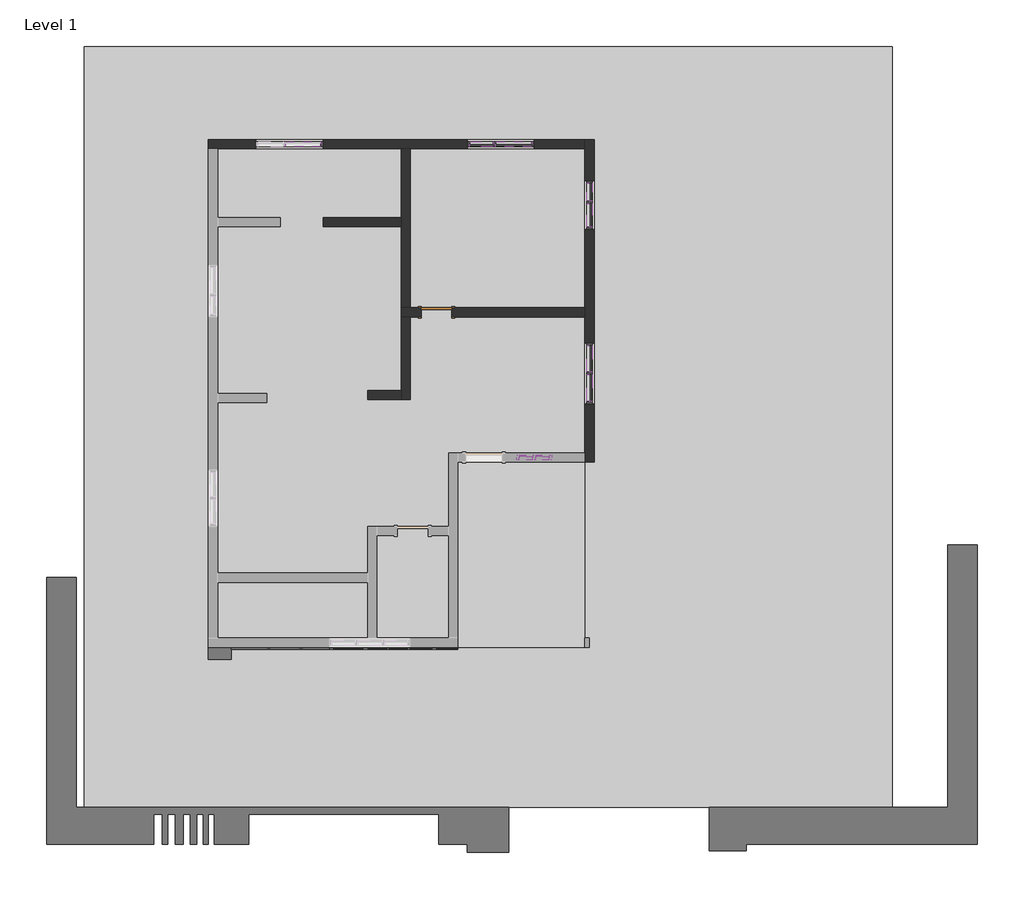
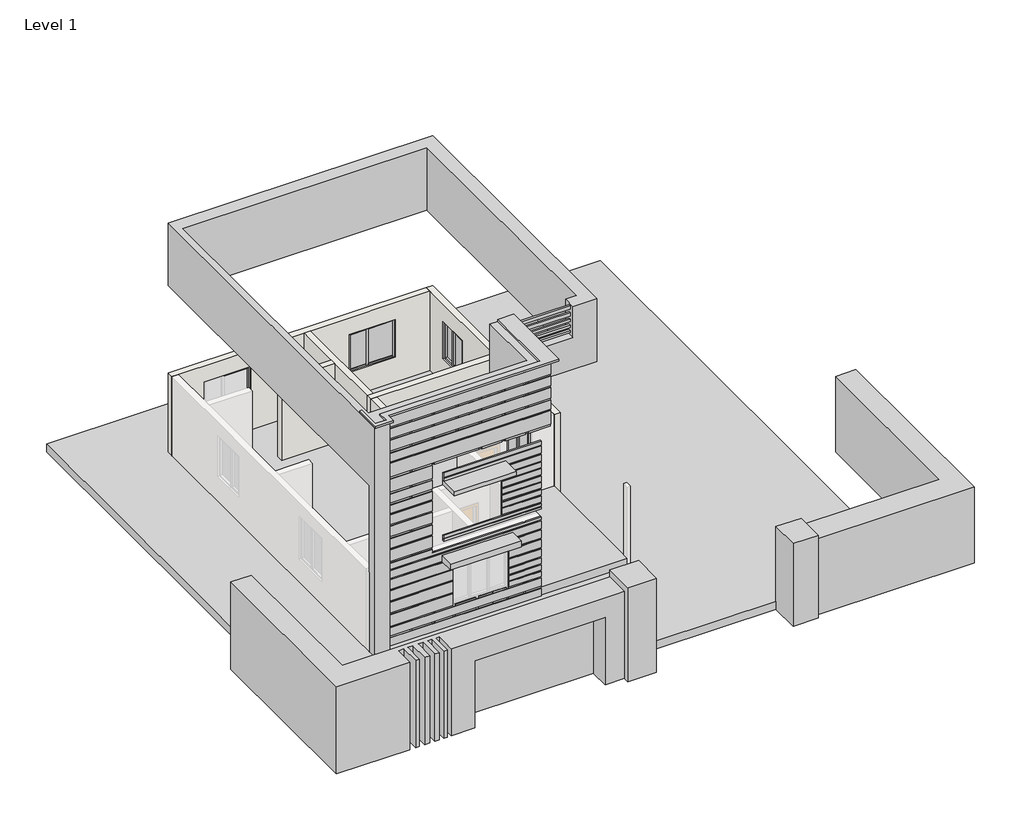
# One storey, part 2 of 2: 30 members, 8 plates, 7 walls, 2 proxies, 1 door.
"""IFC4 building model written with IfcOpenShell, lengths in millimetres."""

from ifc_helpers import new_model, si_unit, origin, origin_with_axes, place, context, project, spatial, polyline, outline, extrude, faceted_brep, transform, mapped, element, save
from components import generic_models_1_generic_models_1_0bf7fa05, generic_models_3_generic_models_3_b56d3d43, generic_models_3_generic_models_3_92db7db1, door_a1484949, member_9f7b9c5b, member_75cd65a6, member_fc57e1ce, member_c33c434a, member_7824d57a, member_cb331184, member_6fb4a552, member_e5d39754, member_b85431e0, member_e39930a5, member_f1f71bde, member_0700671e, member_9dfa5507, member_024c663a, member_55cf8d67, system_panel_glazed_7b9e2e16, system_panel_glazed_a4d37703, system_panel_glazed_197f3525, system_panel_glazed_f1c06e49, system_panel_glazed_593bec76, system_panel_glazed_469e0694

model = new_model("IFC4")

# Units and contexts
model_context = context("Model", 3, world=origin())
ifc_project = project(units=[si_unit("LENGTHUNIT", "METRE", prefix="MILLI")], contexts=[model_context])

# Site, building, storey
site = spatial("IfcSite", under=ifc_project)
building = spatial("IfcBuilding", under=site)
storey = spatial("IfcBuildingStorey", under=building, Name="Level 1", Elevation=0.0)

# Proxies
placement = place(None, origin())
generic_models_1_generic_models_1_shape = generic_models_1_generic_models_1_0bf7fa05(model_context)
element("IfcBuildingElementProxy", 1, Name="Generic Models 1 : Generic Models 1", ObjectType="Generic Models 1 : Generic Models 1", at=placement, inside=storey, context=model_context, shape_type="MappedRepresentation", body=[
    mapped(generic_models_1_generic_models_1_shape, transform((0.0, 0.0, 0.0), x_axis=(1.0, 0.0, 0.0), y_axis=(0.0, 1.0, 0.0), z_axis=(0.0, 0.0, 1.0))),
])
generic_models_3_generic_models_3_shape = generic_models_3_generic_models_3_b56d3d43(model_context)
generic_models_3_generic_models_3_2_shape = generic_models_3_generic_models_3_92db7db1(model_context)
element("IfcBuildingElementProxy", 2, Name="Generic Models 3 : Generic Models 3", ObjectType="Generic Models 3 : Generic Models 3", at=placement, inside=storey, context=model_context, shape_type="MappedRepresentation", body=[
    mapped(generic_models_3_generic_models_3_shape, transform((0.0, 0.0, 0.0), x_axis=(1.0, 0.0, 0.0), y_axis=(0.0, 1.0, 0.0), z_axis=(0.0, 0.0, 1.0))),
    mapped(generic_models_3_generic_models_3_2_shape, transform((0.0, 0.0, 0.0), x_axis=(1.0, 0.0, 0.0), y_axis=(0.0, 1.0, 0.0), z_axis=(0.0, 0.0, 1.0))),
])

# Door
door_shape = door_a1484949(model_context)
element("IfcDoor", 3, ObjectType="Single-Flush : 30\" x 80\"", at=placement, inside=storey, context=model_context, shape_type="MappedRepresentation", body=[
    mapped(door_shape, transform((-12850.1628107, -5472.3642965, 0.0), x_axis=(1.0, 0.0, 0.0), y_axis=(0.0, 1.0, 0.0), z_axis=(0.0, 0.0, 1.0))),
])

# Members
member_shape = member_9f7b9c5b(model_context)
element("IfcMember", 4, ObjectType="Rectangular Mullion : 2.5\" x 5\" rectangular", at=placement, inside=storey, context=model_context, shape_type="MappedRepresentation", body=[
    mapped(member_shape, transform((-10446.6878107, -9091.8642965, 2736.7021457), x_axis=(0.0, 0.0, 1.0), y_axis=(0.0, -1.0, 0.0), z_axis=(1.0, 0.0, 0.0))),
])
element("IfcMember", 5, ObjectType="Rectangular Mullion : 2.5\" x 5\" rectangular", at=placement, inside=storey, context=model_context, shape_type="MappedRepresentation", body=[
    mapped(member_shape, transform((-10037.1128107, -9091.8642965, 2736.7021457), x_axis=(0.0, 0.0, 1.0), y_axis=(0.0, -1.0, 0.0), z_axis=(1.0, 0.0, 0.0))),
])
member_2_shape = member_75cd65a6(model_context)
element("IfcMember", 6, ObjectType="Rectangular Mullion : 2.5\" x 5\" rectangular", at=placement, inside=storey, context=model_context, shape_type="MappedRepresentation", body=[
    mapped(member_2_shape, transform((-10414.9378107, -9091.8642965, 1249.7277266), x_axis=(1.0, 0.0, 0.0), y_axis=(0.0, -1.0, 0.0), z_axis=(0.0, 0.0, -1.0))),
])
element("IfcMember", 7, ObjectType="Rectangular Mullion : 2.5\" x 5\" rectangular", at=placement, inside=storey, context=model_context, shape_type="MappedRepresentation", body=[
    mapped(member_shape, transform((-10383.1878107, -9091.8642965, 1249.7277266), x_axis=(0.0, 0.0, -1.0), y_axis=(0.0, -1.0, 0.0), z_axis=(-1.0, 0.0, 0.0))),
])
element("IfcMember", 8, ObjectType="Rectangular Mullion : 2.5\" x 5\" rectangular", at=placement, inside=storey, context=model_context, shape_type="MappedRepresentation", body=[
    mapped(member_shape, transform((-10792.7628107, -9091.8642965, 1249.7277266), x_axis=(0.0, 0.0, -1.0), y_axis=(0.0, -1.0, 0.0), z_axis=(-1.0, 0.0, 0.0))),
])
member_3_shape = member_fc57e1ce(model_context)
element("IfcMember", 9, ObjectType="Rectangular Mullion : 2.5\" x 5\" rectangular", at=placement, inside=storey, context=model_context, shape_type="MappedRepresentation", body=[
    mapped(member_3_shape, transform((-10856.2628107, -9091.8642965, 2736.7021457), x_axis=(-1.0, 0.0, 0.0), y_axis=(0.0, -1.0, 0.0), z_axis=(0.0, 0.0, 1.0))),
])
element("IfcMember", 10, ObjectType="Rectangular Mullion : 2.5\" x 5\" rectangular", at=placement, inside=storey, context=model_context, shape_type="MappedRepresentation", body=[
    mapped(member_3_shape, transform((-9973.6128107, -9091.8642965, 1249.7277266), x_axis=(1.0, 0.0, 0.0), y_axis=(0.0, -1.0, 0.0), z_axis=(0.0, 0.0, -1.0))),
])
member_4_shape = member_c33c434a(model_context)
element("IfcMember", 11, ObjectType="Rectangular Mullion : 2.5\" x 5\" rectangular", at=placement, inside=storey, context=model_context, shape_type="MappedRepresentation", body=[
    mapped(member_4_shape, transform((-9040.1628107, -7028.1142965, 1098.1511575), x_axis=(0.0, 0.0, -1.0), y_axis=(-1.0, 0.0, 0.0), z_axis=(0.0, 1.0, 0.0))),
])
element("IfcMember", 12, ObjectType="Rectangular Mullion : 2.5\" x 5\" rectangular", at=placement, inside=storey, context=model_context, shape_type="MappedRepresentation", body=[
    mapped(member_4_shape, transform((-9040.1628107, -6297.8642965, 1098.1511575), x_axis=(0.0, 0.0, -1.0), y_axis=(-1.0, 0.0, 0.0), z_axis=(0.0, 1.0, 0.0))),
])
member_5_shape = member_7824d57a(model_context)
element("IfcMember", 13, ObjectType="Rectangular Mullion : 2.5\" x 5\" rectangular", at=placement, inside=storey, context=model_context, shape_type="MappedRepresentation", body=[
    mapped(member_5_shape, transform((-9040.1628107, -6996.3642965, 1098.1511575), x_axis=(0.0, -1.0, 0.0), y_axis=(-1.0, 0.0, 0.0), z_axis=(0.0, 0.0, -1.0))),
])
element("IfcMember", 14, ObjectType="Rectangular Mullion : 2.5\" x 5\" rectangular", at=placement, inside=storey, context=model_context, shape_type="MappedRepresentation", body=[
    mapped(member_4_shape, transform((-9040.1628107, -6964.6142965, 2379.6118359), x_axis=(0.0, 0.0, 1.0), y_axis=(-1.0, 0.0, 0.0), z_axis=(0.0, -1.0, 0.0))),
])
element("IfcMember", 15, ObjectType="Rectangular Mullion : 2.5\" x 5\" rectangular", at=placement, inside=storey, context=model_context, shape_type="MappedRepresentation", body=[
    mapped(member_4_shape, transform((-9040.1628107, -7694.8642965, 2379.6118359), x_axis=(0.0, 0.0, 1.0), y_axis=(-1.0, 0.0, 0.0), z_axis=(0.0, -1.0, 0.0))),
])
member_6_shape = member_cb331184(model_context)
element("IfcMember", 16, ObjectType="Rectangular Mullion : 2.5\" x 5\" rectangular", at=placement, inside=storey, context=model_context, shape_type="MappedRepresentation", body=[
    mapped(member_6_shape, transform((-9040.1628107, -6234.3642965, 2379.6118359), x_axis=(0.0, 1.0, 0.0), y_axis=(-1.0, 0.0, 0.0), z_axis=(0.0, 0.0, 1.0))),
])
element("IfcMember", 17, ObjectType="Rectangular Mullion : 2.5\" x 5\" rectangular", at=placement, inside=storey, context=model_context, shape_type="MappedRepresentation", body=[
    mapped(member_6_shape, transform((-9040.1628107, -7758.3642965, 1098.1511575), x_axis=(0.0, -1.0, 0.0), y_axis=(-1.0, 0.0, 0.0), z_axis=(0.0, 0.0, -1.0))),
])
member_7_shape = member_6fb4a552(model_context)
element("IfcMember", 18, ObjectType="Rectangular Mullion : 2.5\" x 5\" rectangular", at=placement, inside=storey, context=model_context, shape_type="MappedRepresentation", body=[
    mapped(member_7_shape, transform((-9040.1628107, -2259.2642965, 941.1853188), x_axis=(0.0, 0.0, -1.0), y_axis=(-1.0, 0.0, 0.0), z_axis=(0.0, 1.0, 0.0))),
])
member_8_shape = member_e5d39754(model_context)
element("IfcMember", 19, ObjectType="Rectangular Mullion : 2.5\" x 5\" rectangular", at=placement, inside=storey, context=model_context, shape_type="MappedRepresentation", body=[
    mapped(member_8_shape, transform((-9040.1628107, -2760.9142965, 941.1853188), x_axis=(0.0, 0.0, -1.0), y_axis=(-1.0, 0.0, 0.0), z_axis=(0.0, 1.0, 0.0))),
])
element("IfcMember", 20, ObjectType="Rectangular Mullion : 2.5\" x 5\" rectangular", at=placement, inside=storey, context=model_context, shape_type="MappedRepresentation", body=[
    mapped(member_8_shape, transform((-11434.1128107, -1281.3642965, 953.616846), x_axis=(0.0, 0.0, -1.0), y_axis=(0.0, 1.0, 0.0), z_axis=(1.0, 0.0, 0.0))),
])
member_9_shape = member_b85431e0(model_context)
element("IfcMember", 21, ObjectType="Rectangular Mullion : 2.5\" x 5\" rectangular", at=placement, inside=storey, context=model_context, shape_type="MappedRepresentation", body=[
    mapped(member_9_shape, transform((-9040.1628107, -2729.1642965, 941.1853188), x_axis=(0.0, -1.0, 0.0), y_axis=(-1.0, 0.0, 0.0), z_axis=(0.0, 0.0, -1.0))),
])
element("IfcMember", 22, ObjectType="Rectangular Mullion : 2.5\" x 5\" rectangular", at=placement, inside=storey, context=model_context, shape_type="MappedRepresentation", body=[
    mapped(member_7_shape, transform((-9040.1628107, -2697.4142965, 2373.4032942), x_axis=(0.0, 0.0, 1.0), y_axis=(-1.0, 0.0, 0.0), z_axis=(0.0, -1.0, 0.0))),
])
element("IfcMember", 23, ObjectType="Rectangular Mullion : 2.5\" x 5\" rectangular", at=placement, inside=storey, context=model_context, shape_type="MappedRepresentation", body=[
    mapped(member_8_shape, transform((-9040.1628107, -3351.4642965, 2373.4032942), x_axis=(0.0, 0.0, 1.0), y_axis=(-1.0, 0.0, 0.0), z_axis=(0.0, -1.0, 0.0))),
])
element("IfcMember", 24, ObjectType="Rectangular Mullion : 2.5\" x 5\" rectangular", at=placement, inside=storey, context=model_context, shape_type="MappedRepresentation", body=[
    mapped(member_8_shape, transform((-12024.6628107, -1281.3642965, 2408.0133025), x_axis=(0.0, 0.0, 1.0), y_axis=(0.0, 1.0, 0.0), z_axis=(-1.0, 0.0, 0.0))),
])
member_10_shape = member_e39930a5(model_context)
element("IfcMember", 25, ObjectType="Rectangular Mullion : 2.5\" x 5\" rectangular", at=placement, inside=storey, context=model_context, shape_type="MappedRepresentation", body=[
    mapped(member_10_shape, transform((-9040.1628107, -2195.7642965, 2373.4032942), x_axis=(0.0, 1.0, 0.0), y_axis=(-1.0, 0.0, 0.0), z_axis=(0.0, 0.0, 1.0))),
])
element("IfcMember", 26, ObjectType="Rectangular Mullion : 2.5\" x 5\" rectangular", at=placement, inside=storey, context=model_context, shape_type="MappedRepresentation", body=[
    mapped(member_10_shape, transform((-9040.1628107, -3414.9642965, 941.1853188), x_axis=(0.0, -1.0, 0.0), y_axis=(-1.0, 0.0, 0.0), z_axis=(0.0, 0.0, -1.0))),
])
member_11_shape = member_f1f71bde(model_context)
element("IfcMember", 27, ObjectType="Rectangular Mullion : 2.5\" x 5\" rectangular", at=placement, inside=storey, context=model_context, shape_type="MappedRepresentation", body=[
    mapped(member_11_shape, transform((-11370.6128107, -1281.3642965, 2408.0133025), x_axis=(0.0, 0.0, 1.0), y_axis=(0.0, 1.0, 0.0), z_axis=(-1.0, 0.0, 0.0))),
])
member_12_shape = member_0700671e(model_context)
element("IfcMember", 28, ObjectType="Rectangular Mullion : 2.5\" x 5\" rectangular", at=placement, inside=storey, context=model_context, shape_type="MappedRepresentation", body=[
    mapped(member_12_shape, transform((-11402.3628107, -1281.3642965, 953.616846), x_axis=(-1.0, 0.0, 0.0), y_axis=(0.0, 1.0, 0.0), z_axis=(0.0, 0.0, -1.0))),
])
element("IfcMember", 29, ObjectType="Rectangular Mullion : 2.5\" x 5\" rectangular", at=placement, inside=storey, context=model_context, shape_type="MappedRepresentation", body=[
    mapped(member_11_shape, transform((-10475.2628107, -1281.3642965, 953.616846), x_axis=(0.0, 0.0, -1.0), y_axis=(0.0, 1.0, 0.0), z_axis=(1.0, 0.0, 0.0))),
])
member_13_shape = member_9dfa5507(model_context)
element("IfcMember", 30, ObjectType="Rectangular Mullion : 2.5\" x 5\" rectangular", at=placement, inside=storey, context=model_context, shape_type="MappedRepresentation", body=[
    mapped(member_13_shape, transform((-12088.1628107, -1281.3642965, 953.616846), x_axis=(-1.0, 0.0, 0.0), y_axis=(0.0, 1.0, 0.0), z_axis=(0.0, 0.0, -1.0))),
])
element("IfcMember", 31, ObjectType="Rectangular Mullion : 2.5\" x 5\" rectangular", at=placement, inside=storey, context=model_context, shape_type="MappedRepresentation", body=[
    mapped(member_13_shape, transform((-10411.7628107, -1281.3642965, 2408.0133025), x_axis=(1.0, 0.0, 0.0), y_axis=(0.0, 1.0, 0.0), z_axis=(0.0, 0.0, 1.0))),
])
member_14_shape = member_024c663a(model_context)
element("IfcMember", 32, ObjectType="Rectangular Mullion : 2.5\" x 5\" rectangular", at=placement, inside=storey, context=model_context, shape_type="MappedRepresentation", body=[
    mapped(member_14_shape, transform((-15733.0628107, -1281.3642965, 2436.257419), x_axis=(0.0, 0.0, 1.0), y_axis=(0.0, -1.0, 0.0), z_axis=(1.0, 0.0, 0.0))),
])
member_15_shape = member_55cf8d67(model_context)
element("IfcMember", 33, ObjectType="Rectangular Mullion : 2.5\" x 5\" rectangular", at=placement, inside=storey, context=model_context, shape_type="MappedRepresentation", body=[
    mapped(member_15_shape, transform((-15669.5628107, -1281.3642965, 1057.7597182), x_axis=(1.0, 0.0, 0.0), y_axis=(0.0, -1.0, 0.0), z_axis=(0.0, 0.0, -1.0))),
])

# Plates
system_panel_glazed_shape = system_panel_glazed_7b9e2e16(model_context)
element("IfcPlate", 34, ObjectType="System Panel : Glazed", at=placement, inside=storey, context=model_context, shape_type="MappedRepresentation", body=[
    mapped(system_panel_glazed_shape, transform((-10619.7253107, -9091.8642965, 1313.2277266), x_axis=(1.0, 0.0, 0.0), y_axis=(0.0, 1.0, 0.0), z_axis=(0.0, 0.0, 1.0))),
])
element("IfcPlate", 35, ObjectType="System Panel : Glazed", at=placement, inside=storey, context=model_context, shape_type="MappedRepresentation", body=[
    mapped(system_panel_glazed_shape, transform((-10210.1503107, -9091.8642965, 1313.2277266), x_axis=(1.0, 0.0, 0.0), y_axis=(0.0, 1.0, 0.0), z_axis=(0.0, 0.0, 1.0))),
])
system_panel_glazed_2_shape = system_panel_glazed_a4d37703(model_context)
element("IfcPlate", 36, ObjectType="System Panel : Glazed", at=placement, inside=storey, context=model_context, shape_type="MappedRepresentation", body=[
    mapped(system_panel_glazed_2_shape, transform((-9040.1628107, -6631.2392965, 1161.6511575), x_axis=(0.0, -1.0, 0.0), y_axis=(1.0, 0.0, 0.0), z_axis=(0.0, 0.0, 1.0))),
])
element("IfcPlate", 37, ObjectType="System Panel : Glazed", at=placement, inside=storey, context=model_context, shape_type="MappedRepresentation", body=[
    mapped(system_panel_glazed_2_shape, transform((-9040.1628107, -7361.4892965, 1161.6511575), x_axis=(0.0, -1.0, 0.0), y_axis=(1.0, 0.0, 0.0), z_axis=(0.0, 0.0, 1.0))),
])
system_panel_glazed_3_shape = system_panel_glazed_197f3525(model_context)
element("IfcPlate", 38, ObjectType="System Panel : Glazed", at=placement, inside=storey, context=model_context, shape_type="MappedRepresentation", body=[
    mapped(system_panel_glazed_3_shape, transform((-9040.1628107, -2478.3392965, 1004.6853188), x_axis=(0.0, -1.0, 0.0), y_axis=(1.0, 0.0, 0.0), z_axis=(0.0, 0.0, 1.0))),
])
system_panel_glazed_4_shape = system_panel_glazed_f1c06e49(model_context)
element("IfcPlate", 39, ObjectType="System Panel : Glazed", at=placement, inside=storey, context=model_context, shape_type="MappedRepresentation", body=[
    mapped(system_panel_glazed_4_shape, transform((-9040.1628107, -3056.1892965, 1004.6853188), x_axis=(0.0, -1.0, 0.0), y_axis=(1.0, 0.0, 0.0), z_axis=(0.0, 0.0, 1.0))),
])
system_panel_glazed_5_shape = system_panel_glazed_593bec76(model_context)
element("IfcPlate", 40, ObjectType="System Panel : Glazed", at=placement, inside=storey, context=model_context, shape_type="MappedRepresentation", body=[
    mapped(system_panel_glazed_5_shape, transform((-10922.9378107, -1281.3642965, 1017.116846), x_axis=(-1.0, 0.0, 0.0), y_axis=(0.0, -1.0, 0.0), z_axis=(0.0, 0.0, 1.0))),
])
system_panel_glazed_6_shape = system_panel_glazed_469e0694(model_context)
element("IfcPlate", 41, ObjectType="System Panel : Glazed", at=placement, inside=storey, context=model_context, shape_type="MappedRepresentation", body=[
    mapped(system_panel_glazed_6_shape, transform((-11729.3878107, -1281.3642965, 1017.116846), x_axis=(-1.0, 0.0, 0.0), y_axis=(0.0, -1.0, 0.0), z_axis=(0.0, 0.0, 1.0))),
])

# Walls
element("IfcWall", 42, ObjectType="9\"", at=placement, inside=storey, context=model_context, shape_type="Brep", body=[
    faceted_brep([(-9154.4628107, -1167.0642965, 0.0), (-18527.0628107, -1167.0642965, 0.0), (-18527.0628107, -1167.0642965, 3048.0), (-9154.4628107, -1167.0642965, 3048.0), (-10411.7628107, -1167.0642965, 953.616846), (-10411.7628107, -1167.0642965, 2408.0133025), (-12088.1628107, -1167.0642965, 2408.0133025), (-12088.1628107, -1167.0642965, 953.616846), (-17345.9628107, -1167.0642965, 2436.257419), (-17345.9628107, -1167.0642965, 1057.7597182), (-15669.5628107, -1167.0642965, 1057.7597182), (-15669.5628107, -1167.0642965, 2436.257419), (-18527.0628107, -1395.6642965, 0.0), (-18298.4628107, -1395.6642965, 0.0), (-13726.4628107, -1395.6642965, 0.0), (-13497.8628107, -1395.6642965, 0.0), (-9154.4628107, -1395.6642965, 0.0), (-9154.4628107, -1395.6642965, 3048.0), (-13497.8628107, -1395.6642965, 3048.0), (-13726.4628107, -1395.6642965, 3048.0), (-18298.4628107, -1395.6642965, 3048.0), (-18527.0628107, -1395.6642965, 3048.0), (-10411.7628107, -1395.6642965, 2408.0133025), (-10411.7628107, -1395.6642965, 953.616846), (-12088.1628107, -1395.6642965, 953.616846), (-12088.1628107, -1395.6642965, 2408.0133025), (-17345.9628107, -1395.6642965, 1057.7597182), (-17345.9628107, -1395.6642965, 2436.257419), (-15669.5628107, -1395.6642965, 2436.257419), (-15669.5628107, -1395.6642965, 1057.7597182)], [[[0, 1, 2, 3], [4, 5, 6, 7], [8, 9, 10, 11]], [[12, 13, 14, 15, 16, 17, 18, 19, 20, 21], [22, 23, 24, 25], [26, 27, 28, 29]], [[1, 0, 16, 15, 14, 13, 12]], [[3, 2, 21, 20, 19, 18, 17]], [[0, 3, 17, 16]], [[2, 1, 12, 21]], [[22, 5, 4, 23]], [[5, 22, 25, 6]], [[6, 25, 24, 7]], [[23, 4, 7, 24]], [[26, 9, 8, 27]], [[27, 8, 11, 28]], [[28, 11, 10, 29]], [[9, 26, 29, 10]]]),
])
element("IfcWall", 43, ObjectType="9\"", at=placement, inside=storey, context=model_context, shape_type="Brep", body=[
    faceted_brep([(-9154.4628107, -5358.0642965, 0.0), (-12469.1628107, -5358.0642965, 0.0), (-12469.1628107, -5358.0642965, 2032.0), (-13231.1628107, -5358.0642965, 2032.0), (-13231.1628107, -5358.0642965, 0.0), (-13497.8628107, -5358.0642965, 0.0), (-13726.4628107, -5358.0642965, 0.0), (-13726.4628107, -5358.0642965, 3048.0), (-13497.8628107, -5358.0642965, 3048.0), (-9154.4628107, -5358.0642965, 3048.0), (-12469.1628107, -5586.6642965, 2032.0), (-12469.1628107, -5586.6642965, 0.0), (-9154.4628107, -5586.6642965, 0.0), (-9154.4628107, -5586.6642965, 3048.0), (-13497.8628107, -5586.6642965, 3048.0), (-13726.4628107, -5586.6642965, 3048.0), (-13726.4628107, -5586.6642965, 0.0), (-13497.8628107, -5586.6642965, 0.0), (-13231.1628107, -5586.6642965, 0.0), (-13231.1628107, -5586.6642965, 2032.0)], [[[0, 1, 2, 3, 4, 5, 6, 7, 8, 9]], [[10, 11, 12, 13, 14, 15, 16, 17, 18, 19]], [[12, 11, 1, 0]], [[18, 17, 16, 6, 5, 4]], [[9, 8, 7, 15, 14, 13]], [[0, 9, 13, 12]], [[7, 6, 16, 15]], [[2, 1, 11, 10]], [[3, 2, 10, 19]], [[4, 3, 19, 18]]]),
])
element("IfcWall", 44, ObjectType="9\"", at=placement, inside=storey, context=model_context, shape_type="Brep", body=[
    faceted_brep([(-13497.8628107, -5358.0642965, 0.0), (-13497.8628107, -1395.6642965, 0.0), (-13497.8628107, -1395.6642965, 3048.0), (-13497.8628107, -5358.0642965, 3048.0), (-13726.4628107, -5358.0642965, 0.0), (-13726.4628107, -5358.0642965, 3048.0), (-13726.4628107, -3338.7642965, 3048.0), (-13726.4628107, -3110.1642965, 3048.0), (-13726.4628107, -1395.6642965, 3048.0), (-13726.4628107, -1395.6642965, 0.0), (-13726.4628107, -3110.1642965, 0.0), (-13726.4628107, -3338.7642965, 0.0)], [[[0, 1, 2, 3]], [[4, 5, 6, 7, 8, 9, 10, 11]], [[1, 0, 4, 11, 10, 9]], [[3, 2, 8, 7, 6, 5]], [[0, 3, 5, 4]], [[2, 1, 9, 8]]]),
])
element("IfcWall", 45, ObjectType="9\"", at=placement, inside=storey, context=model_context, shape_type="Brep", body=[
    faceted_brep([(-13726.4628107, -5586.6642965, 0.0), (-13726.4628107, -7415.4642965, 0.0), (-13726.4628107, -7644.0642965, 0.0), (-13726.4628107, -7644.0642965, 3048.0), (-13726.4628107, -7415.4642965, 3048.0), (-13726.4628107, -5586.6642965, 3048.0), (-13497.8628107, -5586.6642965, 0.0), (-13497.8628107, -5586.6642965, 3048.0), (-13497.8628107, -7644.0642965, 3048.0), (-13497.8628107, -7644.0642965, 0.0)], [[[0, 1, 2, 3, 4, 5]], [[6, 7, 8, 9]], [[2, 1, 0, 6, 9]], [[5, 4, 3, 8, 7]], [[0, 5, 7, 6]], [[3, 2, 9, 8]]]),
])
element("IfcWall", 46, ObjectType="9\"", at=placement, inside=storey, context=model_context, shape_type="SweptSolid", body=[
    extrude(outline(polyline([(-14564.6628107, -7415.4642965), (-13726.4628107, -7415.4642965), (-13726.4628107, -7644.0642965), (-14564.6628107, -7644.0642965), (-14564.6628107, -7415.4642965)])), origin_with_axes(), (0.0, 0.0, 1.0), 3048.0),
])
element("IfcWall", 47, ObjectType="9\"", at=placement, inside=storey, context=model_context, shape_type="SweptSolid", body=[
    extrude(outline(polyline([(-13726.4628107, -3338.7642965), (-15669.5628107, -3338.7642965), (-15669.5628107, -3110.1642965), (-13726.4628107, -3110.1642965), (-13726.4628107, -3338.7642965)])), origin_with_axes(), (0.0, 0.0, 1.0), 3048.0),
])
element("IfcWall", 48, ObjectType="9\"", at=placement, inside=storey, context=model_context, shape_type="Brep", body=[
    faceted_brep([(-8925.8628107, -9206.1642965, 0.0), (-8925.8628107, -1167.0642965, 0.0), (-8925.8628107, -1167.0642965, 3048.0), (-8925.8628107, -9206.1642965, 3048.0), (-8925.8628107, -6234.3642965, 2379.6118359), (-8925.8628107, -6234.3642965, 1098.1511575), (-8925.8628107, -7758.3642965, 1098.1511575), (-8925.8628107, -7758.3642965, 2379.6118359), (-8925.8628107, -2195.7642965, 2373.4032942), (-8925.8628107, -2195.7642965, 941.1853188), (-8925.8628107, -3414.9642965, 941.1853188), (-8925.8628107, -3414.9642965, 2373.4032942), (-9154.4628107, -1167.0642965, 0.0), (-9154.4628107, -1395.6642965, 0.0), (-9154.4628107, -5358.0642965, 0.0), (-9154.4628107, -5586.6642965, 0.0), (-9154.4628107, -8977.5642965, 0.0), (-9154.4628107, -9206.1642965, 0.0), (-9154.4628107, -9206.1642965, 3048.0), (-9154.4628107, -8977.5642965, 3048.0), (-9154.4628107, -5586.6642965, 3048.0), (-9154.4628107, -5358.0642965, 3048.0), (-9154.4628107, -1395.6642965, 3048.0), (-9154.4628107, -1167.0642965, 3048.0), (-9154.4628107, -6234.3642965, 1098.1511575), (-9154.4628107, -6234.3642965, 2379.6118359), (-9154.4628107, -7758.3642965, 2379.6118359), (-9154.4628107, -7758.3642965, 1098.1511575), (-9154.4628107, -2195.7642965, 941.1853188), (-9154.4628107, -2195.7642965, 2373.4032942), (-9154.4628107, -3414.9642965, 2373.4032942), (-9154.4628107, -3414.9642965, 941.1853188)], [[[0, 1, 2, 3], [4, 5, 6, 7], [8, 9, 10, 11]], [[12, 13, 14, 15, 16, 17, 18, 19, 20, 21, 22, 23], [24, 25, 26, 27], [28, 29, 30, 31]], [[1, 0, 17, 16, 15, 14, 13, 12]], [[3, 2, 23, 22, 21, 20, 19, 18]], [[0, 3, 18, 17]], [[2, 1, 12, 23]], [[24, 5, 4, 25]], [[25, 4, 7, 26]], [[26, 7, 6, 27]], [[5, 24, 27, 6]], [[28, 9, 8, 29]], [[29, 8, 11, 30]], [[30, 11, 10, 31]], [[9, 28, 31, 10]]]),
])

save(model, "model.ifc")

# Revit data of these elements
# Type "Single-Flush : 30\" x 80\""
#   Type Mark = "5"
#   Construction Type Id = "MDOOR"
#   Assembly Code = "C1020"
#   Analytic Construction = "Metal"
#   Thickness = 0' - 2"
#   Heat Transfer Coefficient (U) = 0.651978 BTU/(h·ft²·°F)
#   Height = 6' - 8"
#   Trim Projection Ext = 0' - 1"
#   Trim Projection Int = 0' - 1"
#   Trim Width = 0' - 3"
#   Width = 2' - 6"
#   Define Thermal Properties by = 1
#   Define Thermal Properties by = 1
#   Door Material = Door - Panel
#   Frame Material = Door - Frame
#   Visual Light Transmittance = 0
#   Solar Heat Gain Coefficient = 0
#   Function = (empty or 0)
#   Wall Closure = (empty or 0)
# Type "Rectangular Mullion : 2.5\" x 5\" rectangular"
#   built-in parameter 1007304 = 0.416667 (stored number, unit not read)
#   built-in parameter 1007301 = 0.104167 (stored number, unit not read)
#   built-in parameter 1007300 = 0.104167 (stored number, unit not read)
# Type "System Panel : Glazed"
#   Construction Type Id = "GSP4R"
#   Analytic Construction = "1/8 in Pilkington single glazing"
#   Visual Light Transmittance = 0.9
#   Solar Heat Gain Coefficient = 0.86
#   Heat Transfer Coefficient (U) = 1.18115 BTU/(h·ft²·°F)
#   Define Thermal Properties by = 1
# Type "9\""
#   Assembly Code = "B2010"
#   Layers, outside or top first: 0' - 9" no material (function 1)
# Element 1 (IfcBuildingElementProxy, "Generic Models 1 : Generic Models 1")
#   Phase Created = New Construction
# Element 2 (IfcBuildingElementProxy, "Generic Models 3 : Generic Models 3")
#   Phase Created = New Construction
# Element 3 (IfcDoor, "Single-Flush : 30\" x 80\"")
#   Phase Created = New Construction
#   Materials on its faces: "Door - Frame", "Door - Panel"
# Elements 4, 5, 6, 7, 8, 9, 10, 11, 12, 13, 14, 15, 16, 17, 18, 19, 20, 21, 22, 23, 24, 25, 26, 27, 28, 29, 30, 31, 32, 33 (IfcMember, "Rectangular Mullion : 2.5\" x 5\" rectangular")
#   Phase Created = New Construction
#   Materials on its faces: "Aluminum"
# Elements 34, 35, 36, 37, 38, 39, 40, 41 (IfcPlate, "System Panel : Glazed")
#   Phase Created = New Construction
#   Materials on its faces: "Glass"
# Elements 42, 43, 44, 45, 46, 47, 48 (IfcWall, "9\"")
#   Top Offset = 0' - 0"
#   Base Offset = 0' - 0"
#   Unconnected Height = 10' - 0"
#   wall height = 10' - 0"
#   Phase Created = New Construction
#   Base Constraint = Level 1
#   Materials on its faces: "Default Wall"
# Materials
#   "Door - Panel": class "Wood", colour RGB 210 159 95, transparency 0, Cost = 0
#   "Door - Frame": colour RGB 118 70 51, transparency 0, Cost = 0
#   "Aluminum": class "Metal", colour RGB 247 247 247, transparency 0, Description = "Aluminum 6061", Cost = 0
#   "Glass": class "Glass", colour RGB 0 128 192, transparency 0.75, Description = "Soda Lime Glass", Cost = 0
#   "Default Wall": colour RGB 128 128 128, transparency 0, Cost = 0
